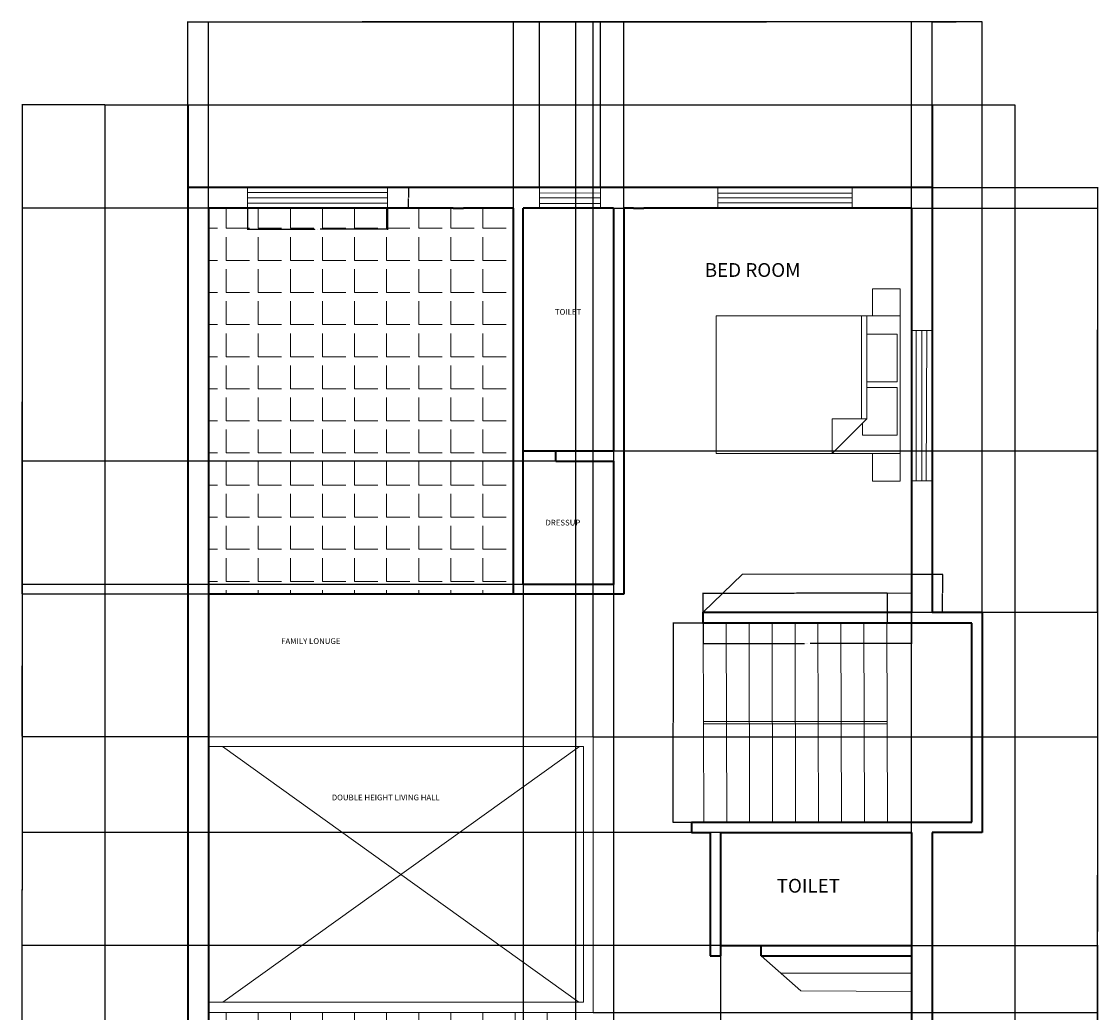
# Model space of a CAD drawing. Units: inches. Extents: x 2621 to 3621, y 1701 to 2465.
# Tile 6 of 6: x 3152 to 3621, y 2034 to 2465. Entities that reach past the tile are written whole.
import ezdxf

# ---------------------------------------------------------------- set-up
doc = ezdxf.new("R2010")
doc.units = ezdxf.units.IN
for name, color, linetype, lineweight in [('A-ANNO-DIMS', 2, 'Continuous', 18), ('A-AREA-IDEN', 7, 'Continuous', 18), ('A-FLOR-CASE', 32, 'Continuous', 18), ('A-FLOR-OPEN', 6, 'Continuous', 18), ('A-FLOR-PATT', 252, 'Continuous', 13), ('A-FLOR-STRS', 30, 'Continuous', 18), ('A-FURN', 8, 'Continuous', 18), ('A-GLAZ', 4, 'Continuous', 18), ('A-WALL', 7, 'Continuous', 35), ('C-PROP', 8, 'Continuous', 25)]:
    doc.layers.add(name, color=color, linetype=linetype, lineweight=lineweight)
doc.styles.get("Standard").update_dxf_attribs({"font": 'arial.ttf'})
doc.dimstyles.get("Standard").update_dxf_attribs({"dimtxt": 0.18, "dimasz": 0.18, "dimexe": 0.18, "dimexo": 0.0625, "dimgap": 0.09, "dimtad": 0, "dimtih": 1, "dimtoh": 1, "dimdec": 4, "dimzin": 0, "dimdsep": 46, "dimtxsty": 'Standard', "dimcen": 0.09, "dimadec": 0, "dimazin": 0, "dimtfac": 1, "dimtdec": 4, "dimtofl": 0, "dimtmove": 0, "dimatfit": 3, "dimfxl": 1, "dimtolj": 1, "dimtzin": 0, "dimarcsym": 0})

# ---------------------------------------------------------------- blocks, each defined once
blk = doc.blocks.new('Bed - Queen')
for p, q in [((0, -80.00003), (0, 0)), ((0, 0), (59.99999, 0)), ((59.99999, 0), (59.99999, -80.00003)), ((7.99999, -1.2), (28.79998, -1.2)), ((7.99999, -14.4), (7.99999, -1.2)), ((28.79998, -1.2), (28.79998, -14.4)), ((31.19999, -1.2), (51.99999, -1.2)), ((31.19999, -14.4), (31.19999, -1.2)), ((51.99999, -1.2), (51.99999, -16.4)), ((0, -14.4), (44.8, -14.4)), ((44.8, -16.8), (0, -16.8)), ((59.99999, -29.6), (44.8, -14.4)), ((44.8, -14.4), (44.8, -29.6)), ((51.99999, -16.4), (46.79936, -16.4)), ((44.8, -29.6), (59.99999, -29.6)), ((59.99999, -80.00003), (0, -80.00003))]:
    blk.add_line(p, q)
blk = doc.blocks.new('LOT-33X57')
for p, q in [((0, 684), (396, 684)), ((0, 0), (0, 684)), ((396, 684), (396, 0)), ((396, 0), (0, 0))]:
    blk.add_line(p, q)
blk = doc.blocks.new('STAIR-RETURN-FLIGHT')
for p, q in [((0.25, 0), (0, 86.58)), ((10.25, 0.03), (10, 86.61)), ((20.25, 0.06), (20, 86.64)), ((30.25, 0.09), (30, 86.67)), ((40.25, 0.12), (40, 86.7)), ((50.25, 0.15), (50, 86.73)), ((60.25, 0.18), (60, 86.76)), ((70.25, 0.2), (70, 86.79)), ((80.25, 0.23), (80, 86.82)), ((6.51, 44.03), (0.13, 44.03)), ((6.51, 43.03), (0.13, 43.03)), ((79.82, 44.03), (6.51, 44.03)), ((79.82, 43.03), (6.51, 43.03)), ((79.82, 44.03), (80.13, 44.03)), ((79.82, 43.03), (80.13, 43.03)), ((70.59, 0.23), (70.59, 0.06))]:
    blk.add_line(p, q)
blk = doc.blocks.new('WIN-65_41')
for p, q in [((2.06, 65.41), (2.06, 0)), ((4.5, 65.41), (4.5, 0)), ((6.45, 0), (6.74, 65.41))]:
    blk.add_line(p, q)
blk.add_lwpolyline([(0, 65.41), (9, 65.41), (9, 0), (0, 0)], close=True)
blk = doc.blocks.new('WIN-60_89')
for p, q in [((0, 6.86), (60.89, 6.86)), ((0, 2.21), (60.89, 2.21))]:
    blk.add_line(p, q)
for points in [[(0, 9), (60.89, 9), (60.89, 0), (0, 0)], [(0, 4.5), (60.89, 4.5), (60.89, 4.5), (0, 4.5)]]:
    blk.add_lwpolyline(points, close=True)
blk = doc.blocks.new('WIN-58_50')
for p, q in [((0, 6.55), (58.5, 6.55)), ((0, 4.5), (58.5, 4.5)), ((0, 2.36), (58.5, 2.36))]:
    blk.add_line(p, q)
blk.add_lwpolyline([(0, 9), (58.5, 9), (58.5, 0), (0, 0)], close=True)
blk = doc.blocks.new('CASEWORK-BEDROOM-WALL-UNIT')
for p, q in [((0, 0), (17.18, 16.58)), ((17.18, 16.58), (90.65, 16.58)), ((8.59, 8.29), (90.65, 8.29))]:
    blk.add_line(p, q)
blk = doc.blocks.new('FURN-BEDSIDE-PAIR')
for points in [[(12, 71.92), (0, 71.92), (0, 83.71), (12, 83.71)], [(12, 11.92), (0, 11.92), (0, 0), (12, 0)]]:
    blk.add_lwpolyline(points, close=True)
blk = doc.blocks.new('*D19')
at = {"layer": 'A-ANNO-DIMS', "color": 0, "lineweight": -2, "transparency": 16777216}
for p, q in [((3448.63, 2203.06), (3435.49, 2203.06)), ((3435.67, 2202.88), (3435.67, 2159.84)), ((3435.67, 2116.42), (3435.67, 2159.47)), ((3448.63, 2116.24), (3435.49, 2116.24))]:
    blk.add_line(p, q, dxfattribs=at)
at = {"layer": 'A-ANNO-DIMS', "color": 0, "transparency": 16777216}
for points in [[(3435.64, 2202.88), (3435.7, 2202.88), (3435.67, 2203.06)], [(3435.64, 2116.42), (3435.7, 2116.42), (3435.67, 2116.24)]]:
    blk.add_solid(points, dxfattribs=at)
at = {"layer": 'Defpoints', "color": 0, "transparency": 16777216}
for p in [(3435.67, 2203.06), (3448.69, 2203.06), (3448.69, 2116.24)]:
    blk.add_point(p, dxfattribs=at)
at = {"layer": 'A-ANNO-DIMS', "color": 0, "transparency": 16777216, "insert": (3435.67, 2159.65), "char_height": 0.18, "attachment_point": 5}
blk.add_mtext('\\A1;FLIGHT 87 TYP.', dxfattribs=at)
blk = doc.blocks.new('*D20')
at = {"layer": 'A-ANNO-DIMS', "color": 0, "lineweight": -2, "transparency": 16777216}
for p, q in [((3448.69, 2203.13), (3448.69, 2216.27)), ((3448.87, 2216.09), (3488.29, 2216.09)), ((3528.76, 2216.09), (3489.34, 2216.09)), ((3528.94, 2203.13), (3528.94, 2216.27))]:
    blk.add_line(p, q, dxfattribs=at)
at = {"layer": 'A-ANNO-DIMS', "color": 0, "transparency": 16777216}
for points in [[(3448.87, 2216.12), (3448.87, 2216.06), (3448.69, 2216.09)], [(3528.76, 2216.12), (3528.76, 2216.06), (3528.94, 2216.09)]]:
    blk.add_solid(points, dxfattribs=at)
at = {"layer": 'Defpoints', "color": 0, "transparency": 16777216}
for p in [(3528.94, 2216.09), (3448.69, 2203.06), (3528.94, 2203.06)]:
    blk.add_point(p, dxfattribs=at)
at = {"layer": 'A-ANNO-DIMS', "color": 0, "transparency": 16777216, "insert": (3488.81, 2216.09), "char_height": 0.18, "attachment_point": 5}
blk.add_mtext('\\A1;80 TYP.', dxfattribs=at)
blk = doc.blocks.new('*D23')
at = {"layer": 'A-ANNO-DIMS', "color": 0, "lineweight": -2, "transparency": 16777216}
for p, q in [((3250.33, 2383.56), (3250.33, 2374.31)), ((3311.23, 2383.56), (3311.23, 2374.31)), ((3250.51, 2374.49), (3279.66, 2374.49)), ((3311.05, 2374.49), (3281.9, 2374.49))]:
    blk.add_line(p, q, dxfattribs=at)
at = {"layer": 'A-ANNO-DIMS', "color": 0, "transparency": 16777216}
for points in [[(3250.51, 2374.52), (3250.51, 2374.46), (3250.33, 2374.49)], [(3311.05, 2374.52), (3311.05, 2374.46), (3311.23, 2374.49)]]:
    blk.add_solid(points, dxfattribs=at)
at = {"layer": 'Defpoints', "color": 0, "transparency": 16777216}
for p in [(3250.33, 2383.63), (3311.23, 2383.63), (3311.23, 2374.49)]:
    blk.add_point(p, dxfattribs=at)
at = {"layer": 'A-ANNO-DIMS', "color": 0, "transparency": 16777216, "insert": (3280.78, 2374.49), "char_height": 0.18, "attachment_point": 5}
blk.add_mtext('\\A1;WINDOW 61 TYP.', dxfattribs=at)
blk = doc.blocks.new('*D24')
at = {"layer": 'A-ANNO-DIMS', "color": 0, "lineweight": -2, "transparency": 16777216}
for p, q in [((3311.29, 2392.63), (3320.54, 2392.63)), ((3320.36, 2392.45), (3320.36, 2388.31)), ((3320.36, 2383.81), (3320.36, 2387.94)), ((3311.29, 2383.63), (3320.54, 2383.63))]:
    blk.add_line(p, q, dxfattribs=at)
at = {"layer": 'A-ANNO-DIMS', "color": 0, "transparency": 16777216}
for points in [[(3320.33, 2392.45), (3320.39, 2392.45), (3320.36, 2392.63)], [(3320.33, 2383.81), (3320.39, 2383.81), (3320.36, 2383.63)]]:
    blk.add_solid(points, dxfattribs=at)
at = {"layer": 'Defpoints', "color": 0, "transparency": 16777216}
for p in [(3311.23, 2392.63), (3320.36, 2392.63), (3311.23, 2383.63)]:
    blk.add_point(p, dxfattribs=at)
at = {"layer": 'A-ANNO-DIMS', "color": 0, "transparency": 16777216, "insert": (3320.36, 2388.13), "char_height": 0.18, "attachment_point": 5}
blk.add_mtext('\\A1;9 TYP.', dxfattribs=at)
blk = doc.blocks.new('*D27')
at = {"layer": 'A-ANNO-DIMS', "color": 0, "lineweight": -2, "transparency": 16777216}
for p, q in [((3448.69, 2207.73), (3448.69, 2194.02)), ((3539.33, 2207.73), (3539.33, 2194.02)), ((3448.87, 2194.2), (3492.77, 2194.2)), ((3539.15, 2194.2), (3495.25, 2194.2))]:
    blk.add_line(p, q, dxfattribs=at)
at = {"layer": 'A-ANNO-DIMS', "color": 0, "transparency": 16777216}
for points in [[(3448.87, 2194.23), (3448.87, 2194.17), (3448.69, 2194.2)], [(3539.15, 2194.23), (3539.15, 2194.17), (3539.33, 2194.2)]]:
    blk.add_solid(points, dxfattribs=at)
at = {"layer": 'Defpoints', "color": 0, "transparency": 16777216}
for p in [(3448.69, 2207.8), (3539.33, 2207.8), (3539.33, 2194.2)]:
    blk.add_point(p, dxfattribs=at)
at = {"layer": 'A-ANNO-DIMS', "color": 0, "transparency": 16777216, "insert": (3494.01, 2194.2), "char_height": 0.18, "attachment_point": 5}
blk.add_mtext('\\A1;WALL UNIT 91 TYP.', dxfattribs=at)
blk = doc.blocks.new('*D28')
at = {"layer": 'A-ANNO-DIMS', "color": 0, "lineweight": -2, "transparency": 16777216}
for p, q in [((3539.4, 2224.38), (3553.11, 2224.38)), ((3552.93, 2224.2), (3552.93, 2216.27)), ((3552.93, 2207.98), (3552.93, 2215.91)), ((3539.4, 2207.8), (3553.11, 2207.8))]:
    blk.add_line(p, q, dxfattribs=at)
at = {"layer": 'A-ANNO-DIMS', "color": 0, "transparency": 16777216}
for points in [[(3552.9, 2224.2), (3552.96, 2224.2), (3552.93, 2224.38)], [(3552.9, 2207.98), (3552.96, 2207.98), (3552.93, 2207.8)]]:
    blk.add_solid(points, dxfattribs=at)
at = {"layer": 'Defpoints', "color": 0, "transparency": 16777216}
for p in [(3539.33, 2224.38), (3552.93, 2224.38), (3539.33, 2207.8)]:
    blk.add_point(p, dxfattribs=at)
at = {"layer": 'A-ANNO-DIMS', "color": 0, "transparency": 16777216, "insert": (3552.93, 2216.09), "char_height": 0.18, "attachment_point": 5}
blk.add_mtext('\\A1;17 TYP.', dxfattribs=at)
blk = doc.blocks.new('*D64')
at = {"layer": 'A-ANNO-DIMS', "color": 0, "lineweight": -2, "transparency": 16777216}
for p, q in [((3188.27, 2428.63), (3152.07, 2428.63)), ((3152.25, 2428.45), (3152.25, 2086.81)), ((3152.25, 1744.81), (3152.25, 2086.44)), ((3188.27, 1744.63), (3152.07, 1744.63))]:
    blk.add_line(p, q, dxfattribs=at)
at = {"layer": 'A-ANNO-DIMS', "color": 0, "transparency": 16777216}
for points in [[(3152.22, 2428.45), (3152.28, 2428.45), (3152.25, 2428.63)], [(3152.22, 1744.81), (3152.28, 1744.81), (3152.25, 1744.63)]]:
    blk.add_solid(points, dxfattribs=at)
at = {"layer": 'Defpoints', "color": 0, "transparency": 16777216}
for p in [(3152.25, 2428.63), (3188.33, 2428.63), (3188.33, 1744.63)]:
    blk.add_point(p, dxfattribs=at)
at = {"layer": 'A-ANNO-DIMS', "color": 0, "transparency": 16777216, "insert": (3152.25, 2086.63), "char_height": 0.18, "attachment_point": 5}
blk.add_mtext('\\A1;684', dxfattribs=at)
blk = doc.blocks.new('*D65')
at = {"layer": 'A-ANNO-DIMS', "color": 0, "lineweight": -2, "transparency": 16777216}
for p, q in [((3224.33, 2428.69), (3224.33, 2464.89)), ((3224.51, 2464.71), (3396.8, 2464.71)), ((3570.01, 2464.71), (3397.72, 2464.71)), ((3570.19, 2207.86), (3570.19, 2464.89))]:
    blk.add_line(p, q, dxfattribs=at)
at = {"layer": 'A-ANNO-DIMS', "color": 0, "transparency": 16777216}
for points in [[(3224.51, 2464.74), (3224.51, 2464.68), (3224.33, 2464.71)], [(3570.01, 2464.74), (3570.01, 2464.68), (3570.19, 2464.71)]]:
    blk.add_solid(points, dxfattribs=at)
at = {"layer": 'Defpoints', "color": 0, "transparency": 16777216}
for p in [(3570.19, 2464.71), (3224.33, 2428.63), (3570.19, 2207.8)]:
    blk.add_point(p, dxfattribs=at)
at = {"layer": 'A-ANNO-DIMS', "color": 0, "transparency": 16777216, "insert": (3397.26, 2464.71), "char_height": 0.18, "attachment_point": 5}
blk.add_mtext('\\A1;345.85', dxfattribs=at)
blk = doc.blocks.new('*D66')
at = {"layer": 'A-ANNO-DIMS', "color": 0, "lineweight": -2, "transparency": 16777216}
for p, q in [((3548.4, 2392.63), (3620.6, 2392.63)), ((3620.42, 2392.45), (3620.42, 2068.81)), ((3620.42, 1744.81), (3620.42, 2068.44)), ((3548.4, 1744.63), (3620.6, 1744.63))]:
    blk.add_line(p, q, dxfattribs=at)
at = {"layer": 'A-ANNO-DIMS', "color": 0, "transparency": 16777216}
for points in [[(3620.39, 2392.45), (3620.45, 2392.45), (3620.42, 2392.63)], [(3620.39, 1744.81), (3620.45, 1744.81), (3620.42, 1744.63)]]:
    blk.add_solid(points, dxfattribs=at)
at = {"layer": 'Defpoints', "color": 0, "transparency": 16777216}
for p in [(3548.33, 2392.63), (3620.42, 2392.63), (3548.33, 1744.63)]:
    blk.add_point(p, dxfattribs=at)
at = {"layer": 'A-ANNO-DIMS', "color": 0, "transparency": 16777216, "insert": (3620.42, 2068.63), "char_height": 0.18, "attachment_point": 5}
blk.add_mtext('\\A1;648', dxfattribs=at)
blk = doc.blocks.new('*D67')
at = {"layer": 'A-ANNO-DIMS', "color": 0, "lineweight": -2, "transparency": 16777216}
for p, q in [((3233.33, 2383.69), (3233.33, 2464.89)), ((3233.51, 2464.71), (3299.26, 2464.71)), ((3365.91, 2464.71), (3300.17, 2464.71)), ((3366.09, 2383.69), (3366.09, 2464.89))]:
    blk.add_line(p, q, dxfattribs=at)
at = {"layer": 'A-ANNO-DIMS', "color": 0, "transparency": 16777216}
for points in [[(3233.51, 2464.74), (3233.51, 2464.68), (3233.33, 2464.71)], [(3365.91, 2464.74), (3365.91, 2464.68), (3366.09, 2464.71)]]:
    blk.add_solid(points, dxfattribs=at)
at = {"layer": 'Defpoints', "color": 0, "transparency": 16777216}
for p in [(3366.09, 2464.71), (3233.33, 2383.63), (3366.09, 2383.63)]:
    blk.add_point(p, dxfattribs=at)
at = {"layer": 'A-ANNO-DIMS', "color": 0, "transparency": 16777216, "insert": (3299.71, 2464.71), "char_height": 0.18, "attachment_point": 5}
blk.add_mtext('\\A1;132.76', dxfattribs=at)
blk = doc.blocks.new('*D68')
at = {"layer": 'A-ANNO-DIMS', "color": 0, "lineweight": -2, "transparency": 16777216}
for p, q in [((3370.34, 2383.56), (3370.34, 1708.36)), ((3409.59, 2383.56), (3409.59, 1708.36)), ((3370.52, 1708.54), (3389.57, 1708.54)), ((3409.41, 1708.54), (3390.36, 1708.54))]:
    blk.add_line(p, q, dxfattribs=at)
at = {"layer": 'A-ANNO-DIMS', "color": 0, "transparency": 16777216}
for points in [[(3370.52, 1708.57), (3370.52, 1708.51), (3370.34, 1708.54)], [(3409.41, 1708.57), (3409.41, 1708.51), (3409.59, 1708.54)]]:
    blk.add_solid(points, dxfattribs=at)
at = {"layer": 'Defpoints', "color": 0, "transparency": 16777216}
for p in [(3370.34, 2383.63), (3409.59, 2383.63), (3409.59, 1708.54)]:
    blk.add_point(p, dxfattribs=at)
at = {"layer": 'A-ANNO-DIMS', "color": 0, "transparency": 16777216, "insert": (3389.97, 1708.54), "char_height": 0.18, "attachment_point": 5}
blk.add_mtext('\\A1;39.25', dxfattribs=at)
blk = doc.blocks.new('*D69')
at = {"layer": 'A-ANNO-DIMS', "color": 0, "lineweight": -2, "transparency": 16777216}
for p, q in [((3414.09, 2383.69), (3414.09, 2464.89)), ((3414.27, 2464.71), (3476.26, 2464.71)), ((3539.15, 2464.71), (3477.17, 2464.71)), ((3539.33, 2383.69), (3539.33, 2464.89))]:
    blk.add_line(p, q, dxfattribs=at)
at = {"layer": 'A-ANNO-DIMS', "color": 0, "transparency": 16777216}
for points in [[(3414.27, 2464.74), (3414.27, 2464.68), (3414.09, 2464.71)], [(3539.15, 2464.74), (3539.15, 2464.68), (3539.33, 2464.71)]]:
    blk.add_solid(points, dxfattribs=at)
at = {"layer": 'Defpoints', "color": 0, "transparency": 16777216}
for p in [(3539.33, 2464.71), (3414.09, 2383.63), (3539.33, 2383.63)]:
    blk.add_point(p, dxfattribs=at)
at = {"layer": 'A-ANNO-DIMS', "color": 0, "transparency": 16777216, "insert": (3476.71, 2464.71), "char_height": 0.18, "attachment_point": 5}
blk.add_mtext('\\A1;125.24', dxfattribs=at)
blk = doc.blocks.new('*D70')
at = {"layer": 'A-ANNO-DIMS', "color": 0, "lineweight": -2, "transparency": 16777216}
for p, q in [((3409.65, 2383.63), (3620.6, 2383.63)), ((3620.42, 2383.45), (3620.42, 2331.05)), ((3620.42, 2278.28), (3620.42, 2330.68)), ((3409.65, 2278.1), (3620.6, 2278.1))]:
    blk.add_line(p, q, dxfattribs=at)
at = {"layer": 'A-ANNO-DIMS', "color": 0, "transparency": 16777216}
for points in [[(3620.39, 2383.45), (3620.45, 2383.45), (3620.42, 2383.63)], [(3620.39, 2278.28), (3620.45, 2278.28), (3620.42, 2278.1)]]:
    blk.add_solid(points, dxfattribs=at)
at = {"layer": 'Defpoints', "color": 0, "transparency": 16777216}
for p in [(3409.59, 2383.63), (3620.42, 2383.63), (3409.59, 2278.1)]:
    blk.add_point(p, dxfattribs=at)
at = {"layer": 'A-ANNO-DIMS', "color": 0, "transparency": 16777216, "insert": (3620.42, 2330.86), "char_height": 0.18, "attachment_point": 5}
blk.add_mtext('\\A1;105.52', dxfattribs=at)
blk = doc.blocks.new('*D71')
at = {"layer": 'A-ANNO-DIMS', "color": 0, "lineweight": -2, "transparency": 16777216}
for p, q in [((3409.53, 2273.6), (3152.07, 2273.6)), ((3152.25, 2273.42), (3152.25, 2246.92)), ((3152.25, 2220.06), (3152.25, 2246.56)), ((3409.53, 2219.88), (3152.07, 2219.88))]:
    blk.add_line(p, q, dxfattribs=at)
at = {"layer": 'A-ANNO-DIMS', "color": 0, "transparency": 16777216}
for points in [[(3152.22, 2273.42), (3152.28, 2273.42), (3152.25, 2273.6)], [(3152.22, 2220.06), (3152.28, 2220.06), (3152.25, 2219.88)]]:
    blk.add_solid(points, dxfattribs=at)
at = {"layer": 'Defpoints', "color": 0, "transparency": 16777216}
for p in [(3152.25, 2273.6), (3409.59, 2273.6), (3409.59, 2219.88)]:
    blk.add_point(p, dxfattribs=at)
at = {"layer": 'A-ANNO-DIMS', "color": 0, "transparency": 16777216, "insert": (3152.25, 2246.74), "char_height": 0.18, "attachment_point": 5}
blk.add_mtext('\\A1;53.73', dxfattribs=at)
blk = doc.blocks.new('*D72')
at = {"layer": 'A-ANNO-DIMS', "color": 0, "lineweight": -2, "transparency": 16777216}
for p, q in [((3233.27, 2383.63), (3152.07, 2383.63)), ((3152.25, 2383.45), (3152.25, 2299.81)), ((3152.25, 2215.81), (3152.25, 2299.44)), ((3233.27, 2215.63), (3152.07, 2215.63))]:
    blk.add_line(p, q, dxfattribs=at)
at = {"layer": 'A-ANNO-DIMS', "color": 0, "transparency": 16777216}
for points in [[(3152.22, 2383.45), (3152.28, 2383.45), (3152.25, 2383.63)], [(3152.22, 2215.81), (3152.28, 2215.81), (3152.25, 2215.63)]]:
    blk.add_solid(points, dxfattribs=at)
at = {"layer": 'Defpoints', "color": 0, "transparency": 16777216}
for p in [(3152.25, 2383.63), (3233.33, 2383.63), (3233.33, 2215.63)]:
    blk.add_point(p, dxfattribs=at)
at = {"layer": 'A-ANNO-DIMS', "color": 0, "transparency": 16777216, "insert": (3152.25, 2299.63), "char_height": 0.18, "attachment_point": 5}
blk.add_mtext('\\A1;168', dxfattribs=at)
blk = doc.blocks.new('*D73')
at = {"layer": 'A-ANNO-DIMS', "color": 0, "lineweight": -2, "transparency": 16777216}
for p, q in [((3233.27, 2215.63), (3152.07, 2215.63)), ((3152.25, 2215.45), (3152.25, 2184.81)), ((3152.25, 2153.81), (3152.25, 2184.44)), ((3233.27, 2153.63), (3152.07, 2153.63))]:
    blk.add_line(p, q, dxfattribs=at)
at = {"layer": 'A-ANNO-DIMS', "color": 0, "transparency": 16777216}
for points in [[(3152.22, 2215.45), (3152.28, 2215.45), (3152.25, 2215.63)], [(3152.22, 2153.81), (3152.28, 2153.81), (3152.25, 2153.63)]]:
    blk.add_solid(points, dxfattribs=at)
at = {"layer": 'Defpoints', "color": 0, "transparency": 16777216}
for p in [(3152.25, 2215.63), (3233.33, 2215.63), (3233.33, 2153.63)]:
    blk.add_point(p, dxfattribs=at)
at = {"layer": 'A-ANNO-DIMS', "color": 0, "transparency": 16777216, "insert": (3152.25, 2184.63), "char_height": 0.18, "attachment_point": 5}
blk.add_mtext('\\A1;62', dxfattribs=at)
blk = doc.blocks.new('*D74')
at = {"layer": 'A-ANNO-DIMS', "color": 0, "lineweight": -2, "transparency": 16777216}
for p, q in [((3233.33, 2153.69), (3233.33, 2464.89)), ((3233.51, 2464.71), (3316.62, 2464.71)), ((3400.63, 2464.71), (3317.53, 2464.71)), ((3400.81, 2153.69), (3400.81, 2464.89))]:
    blk.add_line(p, q, dxfattribs=at)
at = {"layer": 'A-ANNO-DIMS', "color": 0, "transparency": 16777216}
for points in [[(3233.51, 2464.74), (3233.51, 2464.68), (3233.33, 2464.71)], [(3400.63, 2464.74), (3400.63, 2464.68), (3400.81, 2464.71)]]:
    blk.add_solid(points, dxfattribs=at)
at = {"layer": 'Defpoints', "color": 0, "transparency": 16777216}
for p in [(3400.81, 2464.71), (3233.33, 2153.63), (3400.81, 2153.63)]:
    blk.add_point(p, dxfattribs=at)
at = {"layer": 'A-ANNO-DIMS', "color": 0, "transparency": 16777216, "insert": (3317.07, 2464.71), "char_height": 0.18, "attachment_point": 5}
blk.add_mtext('\\A1;167.48', dxfattribs=at)
blk = doc.blocks.new('*D75')
at = {"layer": 'A-ANNO-DIMS', "color": 0, "lineweight": -2, "transparency": 16777216}
for p, q in [((3400.87, 2153.63), (3620.6, 2153.63)), ((3620.42, 2153.45), (3620.42, 2093.81)), ((3620.42, 2033.81), (3620.42, 2093.45)), ((3400.87, 2033.63), (3620.6, 2033.63))]:
    blk.add_line(p, q, dxfattribs=at)
at = {"layer": 'A-ANNO-DIMS', "color": 0, "transparency": 16777216}
for points in [[(3620.39, 2153.45), (3620.45, 2153.45), (3620.42, 2153.63)], [(3620.39, 2033.81), (3620.45, 2033.81), (3620.42, 2033.63)]]:
    blk.add_solid(points, dxfattribs=at)
at = {"layer": 'Defpoints', "color": 0, "transparency": 16777216}
for p in [(3400.81, 2153.63), (3620.42, 2153.63), (3400.81, 2033.63)]:
    blk.add_point(p, dxfattribs=at)
at = {"layer": 'A-ANNO-DIMS', "color": 0, "transparency": 16777216, "insert": (3620.42, 2093.63), "char_height": 0.18, "attachment_point": 5}
blk.add_mtext('\\A1;120', dxfattribs=at)
blk = doc.blocks.new('*D76')
at = {"layer": 'A-ANNO-DIMS', "color": 0, "lineweight": -2, "transparency": 16777216}
for p, q in [((3456.23, 2062.74), (3456.23, 1708.36)), ((3539.33, 2062.74), (3539.33, 1708.36)), ((3456.41, 1708.54), (3497.47, 1708.54)), ((3539.15, 1708.54), (3498.09, 1708.54))]:
    blk.add_line(p, q, dxfattribs=at)
at = {"layer": 'A-ANNO-DIMS', "color": 0, "transparency": 16777216}
for points in [[(3456.41, 1708.57), (3456.41, 1708.51), (3456.23, 1708.54)], [(3539.15, 1708.57), (3539.15, 1708.51), (3539.33, 1708.54)]]:
    blk.add_solid(points, dxfattribs=at)
at = {"layer": 'Defpoints', "color": 0, "transparency": 16777216}
for p in [(3456.23, 2062.8), (3539.33, 2062.8), (3539.33, 1708.54)]:
    blk.add_point(p, dxfattribs=at)
at = {"layer": 'A-ANNO-DIMS', "color": 0, "transparency": 16777216, "insert": (3497.78, 1708.54), "char_height": 0.18, "attachment_point": 5}
blk.add_mtext('\\A1;83.1', dxfattribs=at)
blk = doc.blocks.new('*D77')
at = {"layer": 'A-ANNO-DIMS', "color": 0, "lineweight": -2, "transparency": 16777216}
for p, q in [((3456.17, 2111.98), (3152.07, 2111.98)), ((3152.25, 2111.8), (3152.25, 2087.57)), ((3152.25, 2062.98), (3152.25, 2087.21)), ((3456.17, 2062.8), (3152.07, 2062.8))]:
    blk.add_line(p, q, dxfattribs=at)
at = {"layer": 'A-ANNO-DIMS', "color": 0, "transparency": 16777216}
for points in [[(3152.22, 2111.8), (3152.28, 2111.8), (3152.25, 2111.98)], [(3152.22, 2062.98), (3152.28, 2062.98), (3152.25, 2062.8)]]:
    blk.add_solid(points, dxfattribs=at)
at = {"layer": 'Defpoints', "color": 0, "transparency": 16777216}
for p in [(3152.25, 2111.98), (3456.23, 2111.98), (3456.23, 2062.8)]:
    blk.add_point(p, dxfattribs=at)
at = {"layer": 'A-ANNO-DIMS', "color": 0, "transparency": 16777216, "insert": (3152.25, 2087.39), "char_height": 0.18, "attachment_point": 5}
blk.add_mtext('\\A1;49.18', dxfattribs=at)
blk = doc.blocks.new('*D78')
at = {"layer": 'A-ANNO-DIMS', "color": 0, "lineweight": -2, "transparency": 16777216}
for p, q in [((3393.19, 1925.94), (3393.19, 2464.89)), ((3393.37, 2464.71), (3465.81, 2464.71)), ((3539.15, 2464.71), (3466.72, 2464.71)), ((3539.33, 1930.44), (3539.33, 2464.89))]:
    blk.add_line(p, q, dxfattribs=at)
at = {"layer": 'A-ANNO-DIMS', "color": 0, "transparency": 16777216}
for points in [[(3393.37, 2464.74), (3393.37, 2464.68), (3393.19, 2464.71)], [(3539.15, 2464.74), (3539.15, 2464.68), (3539.33, 2464.71)]]:
    blk.add_solid(points, dxfattribs=at)
at = {"layer": 'Defpoints', "color": 0, "transparency": 16777216}
for p in [(3539.33, 2464.71), (3539.33, 1930.38), (3393.19, 1925.88)]:
    blk.add_point(p, dxfattribs=at)
at = {"layer": 'A-ANNO-DIMS', "color": 0, "transparency": 16777216, "insert": (3466.26, 2464.71), "char_height": 0.18, "attachment_point": 5}
blk.add_mtext('\\A1;146.14', dxfattribs=at)
blk = doc.blocks.new('*D79')
at = {"layer": 'A-ANNO-DIMS', "color": 0, "lineweight": -2, "transparency": 16777216}
for p, q in [((3539.4, 2062.8), (3620.6, 2062.8)), ((3620.42, 2062.62), (3620.42, 1996.77)), ((3620.42, 1930.56), (3620.42, 1996.41)), ((3539.4, 1930.38), (3620.6, 1930.38))]:
    blk.add_line(p, q, dxfattribs=at)
at = {"layer": 'A-ANNO-DIMS', "color": 0, "transparency": 16777216}
for points in [[(3620.39, 2062.62), (3620.45, 2062.62), (3620.42, 2062.8)], [(3620.39, 1930.56), (3620.45, 1930.56), (3620.42, 1930.38)]]:
    blk.add_solid(points, dxfattribs=at)
at = {"layer": 'Defpoints', "color": 0, "transparency": 16777216}
for p in [(3539.33, 2062.8), (3620.42, 2062.8), (3539.33, 1930.38)]:
    blk.add_point(p, dxfattribs=at)
at = {"layer": 'A-ANNO-DIMS', "color": 0, "transparency": 16777216, "insert": (3620.42, 1996.59), "char_height": 0.18, "attachment_point": 5}
blk.add_mtext('\\A1;132.42', dxfattribs=at)
blk = doc.blocks.new('*D103')
at = {"layer": 'A-ANNO-DIMS', "color": 0, "lineweight": -2, "transparency": 16777216}
for p, q in [((3548.33, 2207.86), (3548.33, 2464.89)), ((3548.51, 2464.71), (3558.86, 2464.71)), ((3570.01, 2464.71), (3559.66, 2464.71)), ((3570.19, 2207.86), (3570.19, 2464.89))]:
    blk.add_line(p, q, dxfattribs=at)
at = {"layer": 'A-ANNO-DIMS', "color": 0, "transparency": 16777216}
for points in [[(3548.51, 2464.74), (3548.51, 2464.68), (3548.33, 2464.71)], [(3570.01, 2464.74), (3570.01, 2464.68), (3570.19, 2464.71)]]:
    blk.add_solid(points, dxfattribs=at)
at = {"layer": 'Defpoints', "color": 0, "transparency": 16777216}
for p in [(3570.19, 2464.71), (3548.33, 2207.8), (3570.19, 2207.8)]:
    blk.add_point(p, dxfattribs=at)
at = {"layer": 'A-ANNO-DIMS', "color": 0, "transparency": 16777216, "insert": (3559.26, 2464.71), "char_height": 0.18, "attachment_point": 5}
blk.add_mtext('\\A1;21.85', dxfattribs=at)
blk = doc.blocks.new('*D104')
at = {"layer": 'A-ANNO-DIMS', "color": 0, "lineweight": -2, "transparency": 16777216}
for p, q in [((3539.4, 2383.63), (3620.6, 2383.63)), ((3620.42, 2383.45), (3620.42, 2295.89)), ((3620.42, 2207.98), (3620.42, 2295.53)), ((3539.4, 2207.8), (3620.6, 2207.8))]:
    blk.add_line(p, q, dxfattribs=at)
at = {"layer": 'A-ANNO-DIMS', "color": 0, "transparency": 16777216}
for points in [[(3620.39, 2383.45), (3620.45, 2383.45), (3620.42, 2383.63)], [(3620.39, 2207.98), (3620.45, 2207.98), (3620.42, 2207.8)]]:
    blk.add_solid(points, dxfattribs=at)
at = {"layer": 'Defpoints', "color": 0, "transparency": 16777216}
for p in [(3539.33, 2383.63), (3620.42, 2383.63), (3539.33, 2207.8)]:
    blk.add_point(p, dxfattribs=at)
at = {"layer": 'A-ANNO-DIMS', "color": 0, "transparency": 16777216, "insert": (3620.42, 2295.71), "char_height": 0.18, "attachment_point": 5}
blk.add_mtext('\\A1;175.83', dxfattribs=at)
blk = doc.blocks.new('*D105')
at = {"layer": 'A-ANNO-DIMS', "color": 0, "lineweight": -2, "transparency": 16777216}
for p, q in [((3377.47, 2392.69), (3377.47, 2464.89)), ((3377.65, 2464.71), (3390.31, 2464.71)), ((3403.76, 2464.71), (3391.1, 2464.71)), ((3403.94, 2392.69), (3403.94, 2464.89))]:
    blk.add_line(p, q, dxfattribs=at)
at = {"layer": 'A-ANNO-DIMS', "color": 0, "transparency": 16777216}
for points in [[(3377.65, 2464.74), (3377.65, 2464.68), (3377.47, 2464.71)], [(3403.76, 2464.74), (3403.76, 2464.68), (3403.94, 2464.71)]]:
    blk.add_solid(points, dxfattribs=at)
at = {"layer": 'Defpoints', "color": 0, "transparency": 16777216}
for p in [(3403.94, 2464.71), (3377.47, 2392.63), (3403.94, 2392.63)]:
    blk.add_point(p, dxfattribs=at)
at = {"layer": 'A-ANNO-DIMS', "color": 0, "transparency": 16777216, "insert": (3390.71, 2464.71), "char_height": 0.18, "attachment_point": 5}
blk.add_mtext('\\A1;26.47', dxfattribs=at)

msp = doc.modelspace()

# ---------------------------------------------------------------- hatches: boundary and pattern name
at = {"layer": 'A-FLOR-PATT'}
h = msp.add_hatch(dxfattribs=at)
h.set_pattern_fill('ANGLE', color=256, scale=2)
h.set_pattern_definition([(0, (0, 0), (0, 13.97), [10.16, -3.81]), (90, (0, 0), (-13.97, 9e-16), [10.16, -3.81])])
h.paths.add_polyline_path([(3233.335, 2383.626), (3233.335, 2215.626), (3366.0915, 2215.626), (3366.0915, 2383.626), (3344.3345, 2383.626), (3339.8345, 2383.626)])
h.paths.add_polyline_path([(3233.335, 2033.6278), (3233.335, 1895.6231), (3233.335, 1744.626), (3539.335, 1744.626), (3539.335, 1780.626), (3539.335, 1789.626), (3539.335, 1859.7646), (3539.335, 1862.3069), (3539.335, 1925.8819), (3388.6903, 1925.8819), (3388.6903, 2033.6278)])

# ---------------------------------------------------------------- linework, layer by layer
at = {"layer": 'A-FLOR-CASE'}
for p, q in [((3474.0184, 2058.2992), (3491.1998, 2043.0104)), ((3482.6091, 2050.6548), (3539.335, 2050.6548)), ((3491.1998, 2043.0104), (3539.335, 2042.6834))]:
    msp.add_line(p, q, dxfattribs=at)
at = {"layer": 'A-FLOR-OPEN'}
for p, q in [((3233.4529, 2153.6261), (3233.335, 2153.6261)), ((3233.4529, 2153.6261), (3400.811, 2153.6261)), ((3400.811, 2033.6278), (3400.811, 2153.6261)), ((3233.4529, 2149.3761), (3396.561, 2149.3761)), ((3239.3803, 2149.3761), (3394.535, 2038.1278)), ((3394.8795, 2149.3761), (3239.6154, 2038.1278)), ((3396.561, 2038.1278), (3396.561, 2149.3761)), ((3233.335, 2038.1278), (3396.561, 2038.1278)), ((3233.335, 2033.6278), (3400.811, 2033.6278))]:
    msp.add_line(p, q, dxfattribs=at)
at = {"layer": 'A-GLAZ'}
for p, q in [((3377.4728, 2390.2318), (3403.9447, 2390.2898)), ((3377.4728, 2388.126), (3403.9447, 2388.126)), ((3377.4728, 2385.6574), (3403.9447, 2385.7153))]:
    msp.add_line(p, q, dxfattribs=at)
msp.add_lwpolyline([(3377.4728, 2392.626), (3403.9447, 2392.626), (3403.9447, 2383.626), (3377.4728, 2383.626)], close=True, dxfattribs=at)
at = {"layer": 'A-WALL'}
for p, q in [((3224.335, 2428.626), (3224.335, 1891.1231)), ((3548.335, 2428.626), (3548.335, 2207.7951)), ((3548.335, 2392.626), (3224.335, 2392.626)), ((3233.335, 2383.626), (3233.335, 2171.7953)), ((3339.8345, 2383.626), (3233.335, 2383.626)), ((3339.8345, 2383.626), (3344.3345, 2383.626)), ((3366.0915, 2383.626), (3344.3345, 2383.626)), ((3366.0915, 2215.626), (3366.0915, 2383.626)), ((3409.5915, 2383.626), (3370.3415, 2383.626)), ((3370.3415, 2278.1032), (3370.3415, 2383.626)), ((3409.5915, 2383.626), (3409.5915, 2278.1032)), ((3418.3892, 2383.626), (3414.0915, 2383.626)), ((3414.0915, 2383.626), (3414.0915, 2215.626)), ((3418.3892, 2383.626), (3422.8892, 2383.626)), ((3539.335, 2383.626), (3422.8892, 2383.626)), ((3539.335, 2383.626), (3539.335, 2207.7951)), ((3370.3415, 2278.1032), (3409.5915, 2278.1032)), ((3370.3415, 2273.6032), (3370.3415, 2278.1032)), ((3384.5787, 2273.6032), (3384.5787, 2278.1032)), ((3370.3415, 2219.876), (3370.3415, 2273.6032)), ((3384.5787, 2273.6032), (3409.5915, 2273.6032)), ((3409.5915, 2273.6032), (3409.5915, 2219.876)), ((3409.5915, 2219.876), (3370.3415, 2219.876)), ((3366.0915, 2215.626), (3233.335, 2215.626)), ((3414.0915, 2215.626), (3366.0915, 2215.626)), ((3448.6881, 2207.7951), (3539.335, 2207.7951)), ((3448.6881, 2203.0626), (3448.6881, 2207.7951)), ((3548.335, 2207.7951), (3570.1863, 2207.7951)), ((3570.1863, 2207.7951), (3570.1863, 2111.9772)), ((3455.1966, 2203.0626), (3448.6881, 2203.0626)), ((3448.6881, 2203.0626), (3448.6881, 2203.0626)), ((3448.6881, 2203.0626), (3448.6881, 2202.8284)), ((3565.599, 2203.0626), (3455.1966, 2203.0626)), ((3565.599, 2116.4772), (3565.599, 2203.0626)), ((3233.335, 2171.7953), (3233.335, 2167.2953)), ((3233.335, 2167.2953), (3233.335, 2116.4772)), ((3233.335, 2116.4772), (3233.335, 2111.9772)), ((3443.6477, 2116.4772), (3548.335, 2116.4772)), ((3443.6477, 2116.4772), (3443.6477, 2111.9772)), ((3548.335, 2116.4772), (3565.599, 2116.4772)), ((3233.335, 2111.9772), (3233.335, 1895.6231)), ((3443.6477, 2111.9772), (3451.7276, 2111.9772)), ((3451.7276, 2111.9772), (3451.7276, 2058.2992)), ((3456.2276, 2111.9772), (3456.2276, 2062.7992)), ((3456.2276, 2111.9772), (3539.335, 2111.9772)), ((3539.335, 2111.9772), (3539.335, 2015.622)), ((3548.335, 2111.9772), (3548.335, 1780.626)), ((3570.1863, 2111.9772), (3548.335, 2111.9772)), ((3451.7276, 2058.2992), (3456.2276, 2058.2992)), ((3456.2276, 2062.7992), (3539.335, 2062.7992)), ((3456.2276, 2062.7992), (3456.2276, 2058.2992)), ((3474.0184, 2058.2992), (3474.0184, 2062.7992)), ((3474.0184, 2058.2992), (3539.335, 2058.2992))]:
    msp.add_line(p, q, dxfattribs=at)

# ---------------------------------------------------------------- block references
at = {"layer": 'A-FLOR-CASE'}
msp.add_blockref('CASEWORK-BEDROOM-WALL-UNIT', (3448.6876, 2207.7955), dxfattribs=at)
at = {"layer": 'A-FLOR-STRS'}
msp.add_blockref('STAIR-RETURN-FLIGHT', (3448.6876, 2116.2435), dxfattribs=at)
at = {"layer": 'A-FURN'}
msp.add_blockref('FURN-BEDSIDE-PAIR', (3522.3946, 2264.9205), dxfattribs=at)
at = {"layer": 'A-FURN', "rotation": 270}
msp.add_blockref('Bed - Queen', (3534.3948, 2336.8417), dxfattribs=at)
at = {"layer": 'A-GLAZ'}
for name, p in [('WIN-60_89', (3250.3326, 2383.6265)), ('WIN-58_50', (3455.0146, 2383.6265)), ('WIN-65_41', (3539.3346, 2264.9995))]:
    msp.add_blockref(name, p, dxfattribs=at)
at = {"layer": 'C-PROP'}
msp.add_blockref('LOT-33X57', (3188.3346, 1744.6265), dxfattribs=at)

# ---------------------------------------------------------------- texts
at = {"layer": 'A-AREA-IDEN', "attachment_point": 1}
for s, width, insert, char_height in [('BED ROOM ', 51.297978, (3449.397, 2359.7526), 6), ('TOILET', 2.761486, (3384.1373, 2339.7555), 2.5), ('DRESSUP', 9.225442, (3380.0149, 2248.0595), 2.5), ('FAMILY LONUGE', 83.341811, (3264.9587, 2196.5011), 2.5), ('DOUBLE HEIGHT LIVING HALL', 52.147333, (3286.9992, 2128.4449), 2.5), ('TOILET', 12.444136, (3480.7178, 2091.7755), 6)]:
    msp.add_mtext_dynamic_manual_height_columns(s, width=width, gutter_width=12.5, heights=[0], dxfattribs=dict(at, insert=insert, char_height=char_height))

# ---------------------------------------------------------------- dimensions: what is measured, and where the dimension line sits
at = {"layer": 'A-ANNO-DIMS'}
for base, p1, p2, override, picture, middle in [((3570.1863, 2464.708), (3224.335, 2428.626), (3570.1863, 2207.7951), {"dimdec": 2, "dimlfac": 1, "dimrnd": 0, "dimzin": 0, "dimdsep": 46, "dimlunit": 2}, '*D65', (3397.2606, 2464.708)), ((3366.0915, 2464.708), (3233.335, 2383.626), (3366.0915, 2383.626), {"dimdec": 2, "dimlfac": 1, "dimrnd": 0, "dimzin": 0, "dimdsep": 46, "dimlunit": 2}, '*D67', (3299.7132, 2464.708)), ((3400.811, 2464.708), (3233.335, 2153.6261), (3400.811, 2153.6261), {"dimdec": 2, "dimlfac": 1, "dimrnd": 0, "dimzin": 0, "dimdsep": 46, "dimlunit": 2}, '*D74', (3317.073, 2464.708)), ((3403.9447, 2464.708), (3377.4728, 2392.626), (3403.9447, 2392.626), {"dimdec": 2, "dimlfac": 1, "dimrnd": 0, "dimzin": 0, "dimdsep": 46, "dimlunit": 2}, '*D105', (3390.7088, 2464.708)), ((3539.335, 2464.708), (3393.1903, 1925.8819), (3539.335, 1930.3819), {"dimdec": 2, "dimlfac": 1, "dimrnd": 0, "dimzin": 0, "dimdsep": 46, "dimlunit": 2}, '*D78', (3466.2626, 2464.708)), ((3539.335, 2464.708), (3414.0915, 2383.626), (3539.335, 2383.626), {"dimdec": 2, "dimlfac": 1, "dimrnd": 0, "dimzin": 0, "dimdsep": 46, "dimlunit": 2}, '*D69', (3476.7132, 2464.708)), ((3570.1863, 2464.708), (3548.335, 2207.7951), (3570.1863, 2207.7951), {"dimdec": 2, "dimlfac": 1, "dimrnd": 0, "dimzin": 0, "dimdsep": 46, "dimlunit": 2}, '*D103', (3559.2606, 2464.708)), ((3409.5915, 1708.544), (3370.3415, 2383.626), (3409.5915, 2383.626), {"dimdec": 2, "dimlfac": 1, "dimrnd": 0, "dimzin": 0, "dimdsep": 46, "dimlunit": 2}, '*D68', (3389.9665, 1708.544)), ((3539.335, 1708.544), (3456.2276, 2062.7992), (3539.335, 2062.7992), {"dimdec": 1, "dimlfac": 1, "dimrnd": 0, "dimzin": 0, "dimdsep": 46, "dimlunit": 2}, '*D76', (3497.7813, 1708.544))]:
    dim = msp.add_linear_dim(base=base, p1=p1, p2=p2, dimstyle='Standard', override=override, dxfattribs=at)
    dim.commit()
    dim.dimension.update_dxf_attribs({"geometry": picture, "text_midpoint": middle})
for base, p1, p2, override, picture, middle in [((3152.253, 2428.626), (3188.335, 1744.626), (3188.335, 2428.626), {"dimdec": 0, "dimlfac": 1, "dimrnd": 0, "dimzin": 0, "dimdsep": 46, "dimlunit": 2}, '*D64', (3152.253, 2086.626)), ((3620.417, 2392.626), (3548.335, 1744.626), (3548.335, 2392.626), {"dimdec": 0, "dimlfac": 1, "dimrnd": 0, "dimzin": 0, "dimdsep": 46, "dimlunit": 2}, '*D66', (3620.417, 2068.626)), ((3152.253, 2383.626), (3233.335, 2215.626), (3233.335, 2383.626), {"dimdec": 0, "dimlfac": 1, "dimrnd": 0, "dimzin": 0, "dimdsep": 46, "dimlunit": 2}, '*D72', (3152.253, 2299.626)), ((3620.417, 2383.626), (3409.5915, 2278.1032), (3409.5915, 2383.626), {"dimdec": 2, "dimlfac": 1, "dimrnd": 0, "dimzin": 0, "dimdsep": 46, "dimlunit": 2}, '*D70', (3620.417, 2330.8646)), ((3620.417, 2383.626), (3539.335, 2207.7951), (3539.335, 2383.626), {"dimdec": 2, "dimlfac": 1, "dimrnd": 0, "dimzin": 0, "dimdsep": 46, "dimlunit": 2}, '*D104', (3620.417, 2295.7106)), ((3152.253, 2273.6032), (3409.5915, 2219.876), (3409.5915, 2273.6032), {"dimdec": 2, "dimlfac": 1, "dimrnd": 0, "dimzin": 0, "dimdsep": 46, "dimlunit": 2}, '*D71', (3152.253, 2246.7396)), ((3152.253, 2215.626), (3233.335, 2153.6261), (3233.335, 2215.626), {"dimdec": 0, "dimlfac": 1, "dimrnd": 0, "dimzin": 0, "dimdsep": 46, "dimlunit": 2}, '*D73', (3152.253, 2184.626)), ((3620.417, 2153.6261), (3400.811, 2033.6278), (3400.811, 2153.6261), {"dimdec": 0, "dimlfac": 1, "dimrnd": 0, "dimzin": 0, "dimdsep": 46, "dimlunit": 2}, '*D75', (3620.417, 2093.627)), ((3152.253, 2111.9772), (3456.2276, 2062.7992), (3456.2276, 2111.9772), {"dimdec": 2, "dimlfac": 1, "dimrnd": 0, "dimzin": 0, "dimdsep": 46, "dimlunit": 2}, '*D77', (3152.253, 2087.3882)), ((3620.417, 2062.7992), (3539.335, 1930.3819), (3539.335, 2062.7992), {"dimdec": 2, "dimlfac": 1, "dimrnd": 0, "dimzin": 0, "dimdsep": 46, "dimlunit": 2}, '*D79', (3620.417, 1996.5905))]:
    dim = msp.add_linear_dim(base=base, p1=p1, p2=p2, angle=90, dimstyle='Standard', override=override, dxfattribs=at)
    dim.commit()
    dim.dimension.update_dxf_attribs({"geometry": picture, "text_midpoint": middle})
for base, p1, p2, text, picture, middle in [((3320.3592, 2392.626), (3311.2252, 2383.626), (3311.2252, 2392.626), '<> TYP.', '*D24', (3320.3592, 2388.126)), ((3552.932, 2224.3798), (3539.335, 2207.7951), (3539.335, 2224.3798), '<> TYP.', '*D28', (3552.932, 2216.0875)), ((3435.6651, 2203.0626), (3448.6881, 2116.243), (3448.6881, 2203.0626), 'FLIGHT <> TYP.', '*D19', (3435.6651, 2159.6528))]:
    dim = msp.add_linear_dim(base=base, p1=p1, p2=p2, angle=90, text=text, dimstyle='Standard', override={"dimdec": 0, "dimlfac": 1, "dimrnd": 0, "dimzin": 0, "dimdsep": 46, "dimlunit": 2}, dxfattribs=at)
    dim.commit()
    dim.dimension.update_dxf_attribs({"geometry": picture, "text_midpoint": middle})
for base, p1, p2, text, picture, middle in [((3311.2252, 2374.492), (3250.3322, 2383.626), (3311.2252, 2383.626), 'WINDOW <> TYP.', '*D23', (3280.7787, 2374.492)), ((3528.9412, 2216.0856), (3448.6881, 2203.0626), (3528.9412, 2203.0626), '<> TYP.', '*D20', (3488.8147, 2216.0856)), ((3539.335, 2194.1981), (3448.6881, 2207.7951), (3539.335, 2207.7951), 'WALL UNIT <> TYP.', '*D27', (3494.0115, 2194.1981))]:
    dim = msp.add_linear_dim(base=base, p1=p1, p2=p2, text=text, dimstyle='Standard', override={"dimdec": 0, "dimlfac": 1, "dimrnd": 0, "dimzin": 0, "dimdsep": 46, "dimlunit": 2}, dxfattribs=at)
    dim.commit()
    dim.dimension.update_dxf_attribs({"geometry": picture, "text_midpoint": middle})

doc.saveas('drawing.dxf')
